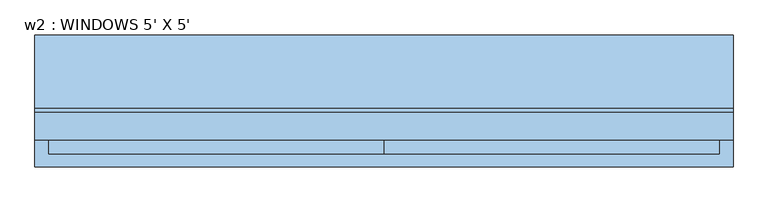
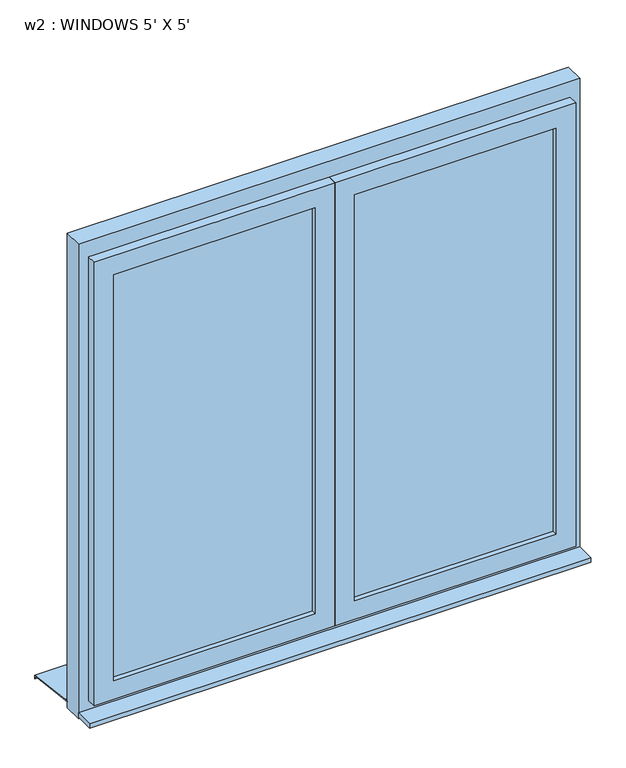
"""IFC4 building model written with IfcOpenShell, lengths in millimetres: window geometry, w2 : WINDOWS 5' X 5'."""

from ifc_helpers import new_model, si_unit, frame, origin, place, context, project, spatial, polyline, outline, extrude, faceted_brep, source, transform, mapped, element, save


def w2_windows_5_x_5_8ac21896(model_context):
    return source(origin(), model_context, "Body", "SolidModel", [
        extrude(outline(polyline([(-15.6778457, 1020.0), (144.3, 1000.0), (144.3, 990.0), (142.3, 990.0), (142.3, 998.3604634), (-15.8759277, 1018.0), (-25.7, 1018.0), (-25.7, 1020.0), (-15.6778457, 1020.0)])), frame((-762.0, 0.0, 0.0), z_axis=(1.0, 0.0, 0.0), x_axis=(0.0, 1.0, 0.0)), (0.0, 0.0, 1.0), 1524.0),
        extrude(outline(polyline([(-762.0, -144.3), (-762.0, -85.7), (762.0, -85.7), (762.0, -144.3), (-762.0, -144.3)])), frame((0.0, 0.0, 1005.0), z_axis=(0.0, 0.0, 1.0), x_axis=(1.0, 0.0, 0.0)), (0.0, 0.0, 1.0), 15.0),
        extrude(outline(polyline([(60.0, -70.7), (672.0, -70.7), (672.0, -100.7), (60.0, -100.7), (60.0, -70.7)])), frame((0.0, 0.0, 1110.0), z_axis=(0.0, 0.0, 1.0), x_axis=(1.0, 0.0, 0.0)), (0.0, 0.0, 1.0), 1304.0),
        extrude(outline(polyline([(-672.0, -70.7), (-60.0, -70.7), (-60.0, -100.7), (-672.0, -100.7), (-672.0, -70.7)])), frame((0.0, 0.0, 1110.0), z_axis=(0.0, 0.0, 1.0), x_axis=(1.0, 0.0, 0.0)), (0.0, 0.0, 1.0), 1304.0),
        extrude(outline(polyline([(2524.0, -762.0), (1000.0, -762.0), (1000.0, 762.0), (2524.0, 762.0), (2524.0, -762.0)]), holes=[polyline([(2444.0, -702.0), (2444.0, 702.0), (1080.0, 702.0), (1080.0, -702.0), (2444.0, -702.0)])]), frame((0.0, -85.7, 0.0), z_axis=(0.0, 1.0, 0.0), x_axis=(0.0, 0.0, 1.0)), (0.0, 0.0, 1.0), 60.0),
        extrude(outline(polyline([(30.0, -85.7), (-30.0, -85.7), (-30.0, -25.7), (30.0, -25.7), (30.0, -85.7)])), frame((0.0, 0.0, 1080.0), z_axis=(0.0, 0.0, 1.0), x_axis=(1.0, 0.0, 0.0)), (0.0, 0.0, 1.0), 1364.0),
        faceted_brep([(30.0, -85.7, 1080.0), (30.0, -55.7, 1080.0), (702.0, -55.7, 1080.0), (702.0, -85.7, 1080.0), (702.0, -55.7, 2444.0), (702.0, -85.7, 2444.0), (30.0, -55.7, 2444.0), (672.0, -55.7, 2414.0), (60.0, -55.7, 2414.0), (60.0, -55.7, 1110.0), (672.0, -55.7, 1110.0), (732.0, -85.7, 1050.0), (0.0, -85.7, 1050.0), (0.0, -85.7, 2474.0), (732.0, -85.7, 2474.0), (30.0, -85.7, 2444.0), (0.0, -115.7, 1050.0), (732.0, -115.7, 1050.0), (732.0, -115.7, 2474.0), (0.0, -115.7, 2474.0), (672.0, -115.7, 1110.0), (60.0, -115.7, 1110.0), (60.0, -115.7, 2414.0), (672.0, -115.7, 2414.0)], [[[0, 1, 2, 3]], [[3, 2, 4, 5]], [[2, 1, 6, 4], [7, 8, 9, 10]], [[11, 12, 13, 14], [5, 15, 0, 3]], [[16, 12, 11, 17]], [[17, 11, 14, 18]], [[18, 19, 16, 17], [20, 21, 22, 23]], [[9, 21, 20, 10]], [[10, 20, 23, 7]], [[15, 6, 1, 0]], [[19, 13, 12, 16]], [[8, 22, 21, 9]], [[5, 4, 6, 15]], [[18, 14, 13, 19]], [[7, 23, 22, 8]]]),
        faceted_brep([(-702.0, -85.7, 1080.0), (-702.0, -55.7, 1080.0), (-30.0, -55.7, 1080.0), (-30.0, -85.7, 1080.0), (-30.0, -55.7, 2444.0), (-30.0, -85.7, 2444.0), (-702.0, -55.7, 2444.0), (-60.0, -55.7, 2414.0), (-672.0, -55.7, 2414.0), (-672.0, -55.7, 1110.0), (-60.0, -55.7, 1110.0), (0.0, -85.7, 1050.0), (-732.0, -85.7, 1050.0), (-732.0, -85.7, 2474.0), (0.0, -85.7, 2474.0), (-702.0, -85.7, 2444.0), (-732.0, -115.7, 1050.0), (0.0, -115.7, 1050.0), (0.0, -115.7, 2474.0), (-732.0, -115.7, 2474.0), (-60.0, -115.7, 1110.0), (-672.0, -115.7, 1110.0), (-672.0, -115.7, 2414.0), (-60.0, -115.7, 2414.0)], [[[0, 1, 2, 3]], [[3, 2, 4, 5]], [[2, 1, 6, 4], [7, 8, 9, 10]], [[11, 12, 13, 14], [5, 15, 0, 3]], [[16, 12, 11, 17]], [[17, 11, 14, 18]], [[18, 19, 16, 17], [20, 21, 22, 23]], [[9, 21, 20, 10]], [[10, 20, 23, 7]], [[15, 6, 1, 0]], [[19, 13, 12, 16]], [[8, 22, 21, 9]], [[5, 4, 6, 15]], [[18, 14, 13, 19]], [[7, 23, 22, 8]]]),
    ])


if __name__ == "__main__":
    model = new_model("IFC4")
    model_context = context("Model", 3, world=origin())
    ifc_project = project(units=[si_unit("LENGTHUNIT", "METRE", prefix="MILLI")], contexts=[model_context])
    site = spatial("IfcSite", under=ifc_project)
    building = spatial("IfcBuilding", under=site)
    placement = place(None, origin())
    w2_windows_5_x_5_shape = w2_windows_5_x_5_8ac21896(model_context)
    element("IfcWindow", 1, ObjectType="w2 : WINDOWS 5' X 5'", at=placement, inside=building, context=model_context, shape_type="MappedRepresentation", body=[
        mapped(w2_windows_5_x_5_shape, transform((0.0, 0.0, 0.0), x_axis=(1.0, 0.0, 0.0), y_axis=(0.0, 1.0, 0.0), z_axis=(0.0, 0.0, 1.0))),
    ])
    save(model, "model.ifc")

# Revit data of these elements
# Type "w2 : WINDOWS 5' X 5'"
#   Type Mark = "26"
#   Operation = "DoublePanelVertical"
#   Keynote = "16.05.01"
#   Analytic Construction = "<None>"
#   Rough Width = 5' - 0"
#   Rough Height = 5' - 0"
#   Rahmentiefe = 0' - 2.3622"
#   Rahmenhöhe unten = 0' - 3.14961"
#   Rahmehöhe oben = 0' - 3.14961"
#   Rahmenbreite = 0' - 2.3622"
#   Heat Transfer Coefficient (U) = 2.81836 BTU/(h·ft²·°F)
#   Height = 5' - 0"
#   Flügeltiefe = 0' - 2.3622"
#   Flügelbreite = 0' - 2.3622"
#   Einbautiefe (von außen) [instance default] = 0' - 5.51181"
#   Width = 5' - 0"
#   Kippflügel [instance default] = yes
#   Drehflügel im Grundriß darstellen [instance default] = no
#   Drehflügel [instance default] = yes
#   Define Thermal Properties by = 1
#   Rahmen [instance default] = none
#   Glas [instance default] = blue glass
#   Flügel [instance default] = WINDOW COLOUR WHITE
#   Fensterbank aussen [instance default] = WINDOW COLOUR WHITE
#   Fensterbank innen [instance default] = WINDOW COLOUR WHITE
#   Visual Light Transmittance = 0
#   Thermal Resistance (R) = 0
#   Solar Heat Gain Coefficient = 0
#   Wall Closure = (empty or 0)
# Element 1 (IfcWindow, "w2 : WINDOWS 5' X 5'")
#   Materials on its faces: "WINDOW COLOUR WHITE", "blue glass"
# Materials
#   "blue glass": class "System", colour RGB 0 0 255, transparency 0.75, Cost = 0
#   "WINDOW COLOUR WHITE": class "Generic", colour RGB 120 120 120, transparency 0, Cost = 0
